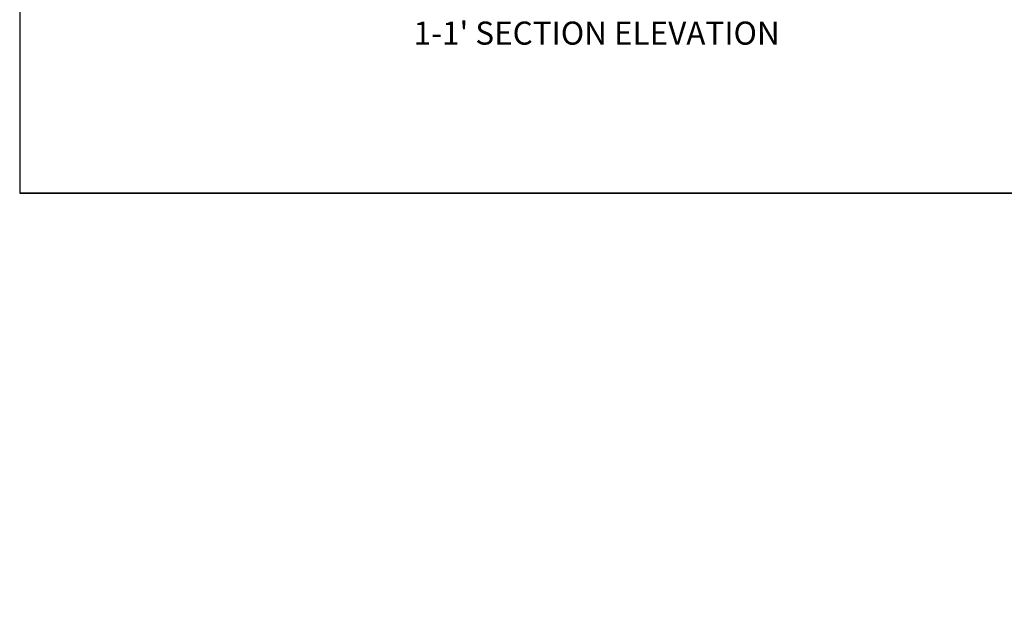
# Model space of a CAD drawing. Units: millimetres. Extents: x 20768 to 23556, y 50760 to 52704.
# Tile 1 of 36: x 20768 to 21280, y 50760 to 51066. Entities that reach past the tile are written whole.
import ezdxf

# ---------------------------------------------------------------- set-up
doc = ezdxf.new("R2010")
doc.units = ezdxf.units.MM
for name, color, linetype, lineweight in [('A-ANNO-TEXT', 7, 'Continuous', 18), ('A-ANNO-TTLB', 7, 'Continuous', 35), ('A-ELEV', 7, 'Continuous', 25), ('A-ELEV-PATT', 8, 'Continuous', 13)]:
    doc.layers.add(name, color=color, linetype=linetype, lineweight=lineweight)
doc.styles.get("Standard").update_dxf_attribs({"font": 'arial.ttf'})

msp = doc.modelspace()

# ---------------------------------------------------------------- hatches: boundary and pattern name
at = {"layer": 'A-ELEV-PATT'}
h = msp.add_hatch(dxfattribs=at)
h.set_pattern_fill('AR-CONC', color=256, scale=8)
h.paths.add_polyline_path([(21106.86, 51149.66), (21094.86, 51149.66), (21094.86, 51077.66), (21022.86, 51077.66), (21022.86, 51149.66), (21016.86, 51149.66), (21016.86, 51077.66), (20866.86, 51077.66), (20866.86, 50768.86), (20854.86, 50768.86), (20854.86, 50759.86), (20890.86, 50759.86), (20890.86, 50768.86), (20878.86, 50768.86), (20878.86, 50807.86), (21016.86, 50807.86), (21016.86, 50768.86), (21007.86, 50768.86), (21007.86, 50759.86), (21031.86, 50759.86), (21031.86, 50768.86), (21022.86, 50768.86), (21022.86, 50807.86), (21094.86, 50807.86), (21094.86, 50768.86), (21082.86, 50768.86), (21082.86, 50759.86), (21118.86, 50759.86), (21118.86, 50768.86), (21106.86, 50768.86)])
h.paths.add_polyline_path([(21022.86, 50939.76), (21094.86, 50939.76), (21094.86, 50813.86), (21022.86, 50813.86)], flags=16)
h.paths.add_polyline_path([(21016.86, 50939.76), (21016.86, 50813.86), (20878.86, 50813.86), (20878.86, 50939.76)], flags=16)
h.paths.add_polyline_path([(21022.86, 50945.76), (21022.86, 51071.66), (21094.86, 51071.66), (21094.86, 50945.76)], flags=16)
h.paths.add_polyline_path([(21016.86, 50945.76), (20878.86, 50945.76), (20878.86, 51071.66), (21016.86, 51071.66)], flags=16)
h.paths.add_polyline_path([(20957.01, 51017.76), (20957.01, 51020.76), (21012.86, 51020.76), (21012.86, 51017.76)], flags=0)
h.paths.add_polyline_path([(21005.86, 50980.26), (20984.86, 50945.76), (20963.86, 50980.26), (20963.86, 51014.76), (21005.86, 51014.76)], flags=0)
h.paths.add_polyline_path([(20963.86, 50980.26), (20984.86, 51014.76), (21005.86, 50980.26)], flags=0)
h.paths.add_polyline_path([(21030.86, 50980.26), (21030.86, 51027.36), (21061.56, 51027.36), (21061.56, 50980.26)], flags=0)
h.paths.add_polyline_path([(21032.86, 50982.26), (21032.86, 51010.26), (21059.56, 51010.26), (21059.56, 50982.26)], flags=0)
h.paths.add_polyline_path([(21034.86, 50984.26), (21034.86, 51008.26), (21045.21, 51008.26), (21045.21, 50984.26)], flags=0)
h.paths.add_polyline_path([(21030.86, 50895.46), (21061.56, 50895.46), (21061.56, 50848.36), (21030.86, 50848.36)], flags=0)
h.paths.add_polyline_path([(21032.86, 50893.46), (21059.56, 50893.46), (21059.56, 50880.36), (21032.86, 50880.36)], flags=0)
h.paths.add_polyline_path([(21047.21, 50984.26), (21047.21, 51008.26), (21057.56, 51008.26), (21057.56, 50984.26)], flags=0)
h.paths.add_polyline_path([(20989.07, 50982.94), (20988.43, 50982.94, -0.960515), (20986.68, 50983.01, -0.414214), (20987.56, 50983.89), (20987.56, 50984.45, -0.357901), (20987.34, 50984.72, -1), (20987.88, 50984.72, -0.34824), (20987.67, 50984.45), (20987.67, 50983.88, -0.376216), (20988.43, 50983.01), (20989.07, 50983.01)], flags=0)
h.paths.add_polyline_path([(21012.86, 50888.86), (21012.86, 50885.86), (20957.01, 50885.86), (20957.01, 50888.86)], flags=0)
h.paths.add_polyline_path([(20981.29, 50982.94), (20980.65, 50982.94), (20980.65, 50983.01), (20981.28, 50983.01, -0.376216), (20982.04, 50983.88), (20982.04, 50984.45, -0.34824), (20981.83, 50984.72, -1), (20982.38, 50984.72, -0.357901), (20982.16, 50984.45), (20982.16, 50983.89, -0.414214), (20983.04, 50983.01, -0.960515)], flags=0)
h.paths.add_polyline_path([(21005.86, 50882.86), (21005.86, 50848.36), (20984.86, 50813.86), (20963.86, 50848.36), (20963.86, 50882.86)], flags=0)
h.paths.add_polyline_path([(21032.86, 50878.36), (21059.56, 50878.36), (21059.56, 50850.36), (21032.86, 50850.36)], flags=0)
h.paths.add_polyline_path([(21034.86, 50876.36), (21045.21, 50876.36), (21045.21, 50852.36), (21034.86, 50852.36)], flags=0)
h.paths.add_polyline_path([(20984.86, 50882.86), (21005.86, 50848.36), (20963.86, 50848.36)], flags=0)
h.paths.add_polyline_path([(20950.86, 50825.86), (20914.86, 50825.86), (20914.86, 50873.86), (20950.86, 50873.86)], flags=0)
h.paths.add_polyline_path([(20950.86, 50957.76), (20914.86, 50957.76), (20914.86, 51005.76), (20950.86, 51005.76)], flags=0)
h.paths.add_polyline_path([(21047.21, 50876.36), (21057.56, 50876.36), (21057.56, 50852.36), (21047.21, 50852.36)], flags=0)
h.paths.add_polyline_path([(21032.86, 51012.26), (21032.86, 51025.36), (21059.56, 51025.36), (21059.56, 51012.26)], flags=0)
h.paths.add_polyline_path([(20987.88, 50852.82, -0.34824), (20987.67, 50852.55), (20987.67, 50851.98, -0.376216), (20988.43, 50851.11), (20989.07, 50851.11), (20989.07, 50851.04), (20988.43, 50851.04, -0.960515), (20986.68, 50851.11, -0.414214), (20987.56, 50851.99), (20987.56, 50852.55, -0.357901), (20987.34, 50852.82, -1)], flags=0)
h.paths.add_polyline_path([(20982.38, 50852.82, -0.357901), (20982.16, 50852.55), (20982.16, 50851.99, -0.414214), (20983.04, 50851.11, -0.960515), (20981.29, 50851.04), (20980.65, 50851.04), (20980.65, 50851.11), (20981.28, 50851.11, -0.376216), (20982.04, 50851.98), (20982.04, 50852.55, -0.34824), (20981.83, 50852.82, -1)], flags=0)

# ---------------------------------------------------------------- linework, layer by layer
at = {"layer": 'A-ANNO-TTLB'}
msp.add_line((20768.14, 50975.78), (22719.7, 50975.78), dxfattribs=at)
at = {"layer": 'A-ELEV'}
msp.add_line((20768.14, 51623.53), (20768.14, 50975.78), dxfattribs=at)

# ---------------------------------------------------------------- texts
at = {"layer": 'A-ANNO-TEXT', "insert": (20965.61, 51064.92), "char_height": 12, "attachment_point": 1}
msp.add_mtext_dynamic_manual_height_columns("  1-1' SECTION ELEVATION", width=241.5904, gutter_width=12.5, heights=[0], dxfattribs=at)

doc.saveas('drawing.dxf')
